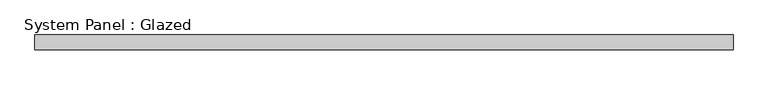
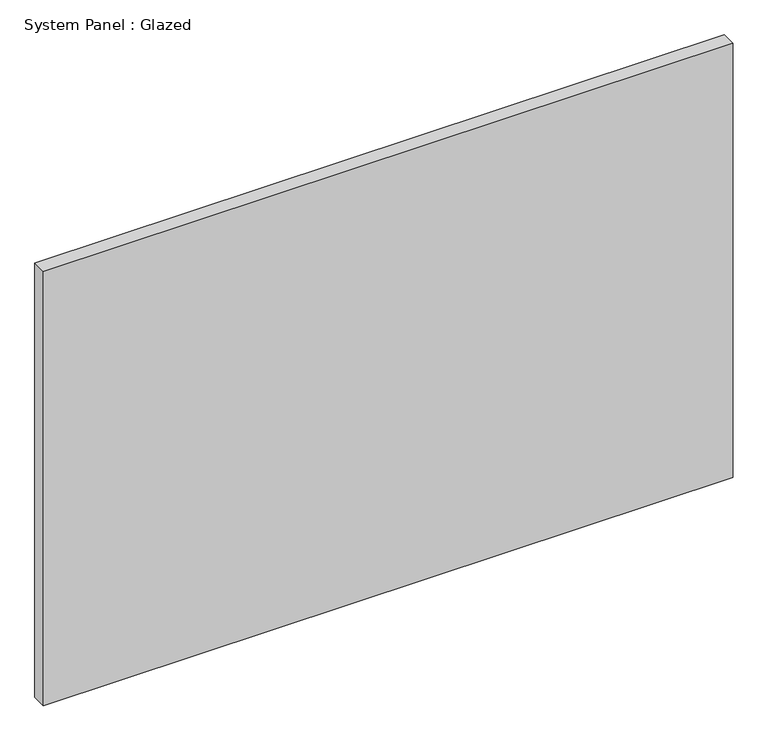
"""IFC4 building model written with IfcOpenShell, lengths in millimetres: plate geometry, System Panel : Glazed."""

from ifc_helpers import new_model, si_unit, origin, origin_with_axes, place, context, project, spatial, polyline, outline, extrude, source, transform, mapped, element, save


def system_panel_glazed_66c18ae2(model_context):
    return source(origin(), model_context, "Body", "SweptSolid", [
        extrude(outline(polyline([(588.8199353, 19.05), (-588.8199353, 19.05), (-588.8199353, 44.45), (588.8199353, 44.45), (588.8199353, 19.05)])), origin_with_axes(), (0.0, 0.0, 1.0), 784.5104839),
    ])


if __name__ == "__main__":
    model = new_model("IFC4")
    model_context = context("Model", 3, world=origin())
    ifc_project = project(units=[si_unit("LENGTHUNIT", "METRE", prefix="MILLI")], contexts=[model_context])
    site = spatial("IfcSite", under=ifc_project)
    building = spatial("IfcBuilding", under=site)
    placement = place(None, origin())
    system_panel_glazed_shape = system_panel_glazed_66c18ae2(model_context)
    element("IfcPlate", 1, ObjectType="System Panel : Glazed", at=placement, inside=building, context=model_context, shape_type="MappedRepresentation", body=[
        mapped(system_panel_glazed_shape, transform((0.0, 0.0, 0.0), x_axis=(1.0, 0.0, 0.0), y_axis=(0.0, 1.0, 0.0), z_axis=(0.0, 0.0, 1.0))),
    ])
    save(model, "model.ifc")

# Revit data of these elements
# Type "System Panel : Glazed"
#   Construction Type Id = "GSP4R"
#   Analytic Construction = "1/8 in Pilkington single glazing"
#   Visual Light Transmittance = 0.9
#   Solar Heat Gain Coefficient = 0.86
#   Heat Transfer Coefficient (U) = 1.18115 BTU/(h·ft²·°F)
#   Define Thermal Properties by = 1
# Element 1 (IfcPlate, "System Panel : Glazed")
#   Materials on its faces: "Glass"
# Materials
#   "Glass": class "Glass", colour RGB 0 128 192, transparency 0.75, Description = "Soda Lime Glass", Cost = 0
